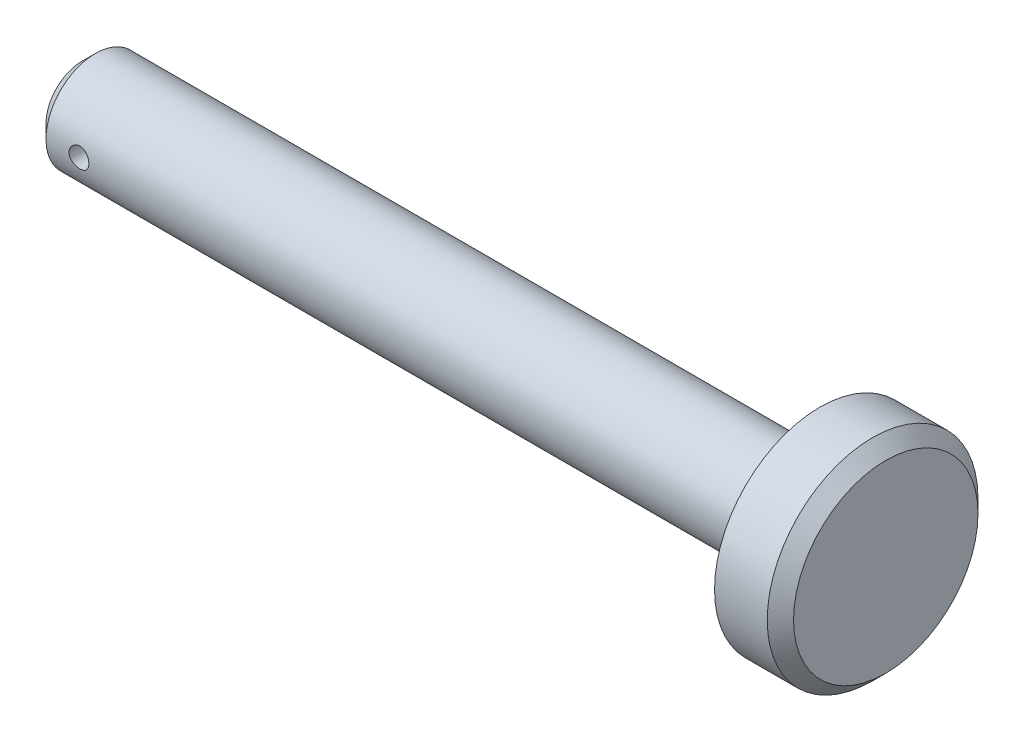
SolidWorks part; units mm, degrees
material "Plain Carbon Steel"
ref_plane "Front Plane" through (0, 0, 0) normal (0, 0, 1) x (1, 0, 0)
ref_plane "Top Plane" through (0, 0, 0) normal (0, 1, 0) x (1, 0, 0)
ref_plane "Right Plane" through (0, 0, 0) normal (1, 0, 0) x (0, 0, -1)
sketch "Pin Profile Sketch" plane through (0, 0, 0) normal (0, 0, 1) x (1, 0, 0)
  line L0 (0, -7.5) -> (112, -7.5)
  line L1 (112, -7.5) -> (112, -16)
  line L2 (112, -16) -> (122, -16)
  line L3 (122, -16) -> (122, 0)
  line L4 (122, 0) -> (0, 0)
  line L5 (0, 0) -> (0, -7.5)
  dimension "D1" = 7.5
  dimension "D2" = 16
  dimension "D3" = 112
  dimension "D4" = 10
revolve "Pin Body" add sketch "Pin Profile Sketch" angle 360 about L4
sketch "Cross Hole Sketch" plane through (0, 0, 0) normal (0, 0, 1) x (1, 0, 0)
  line L0 (112, 16) -> (112, -16) construction
  circle A0 centre (7, 0) radius 1.5
  dimension "D1" = 3
  dimension "D2" = 105
extrude "Cross Hole Ø3" cut sketch "Cross Hole Sketch" against normal through all both and the other way through all
chamfer "Chamfer 2x45°" distance 2 angle 45 2 edges at (0, 7.5, 0) (122, 16, 0)
